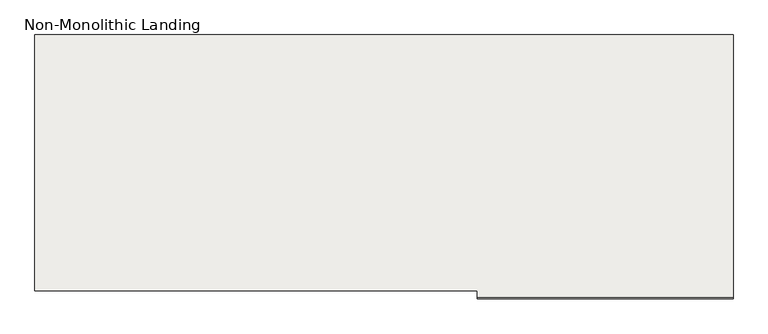
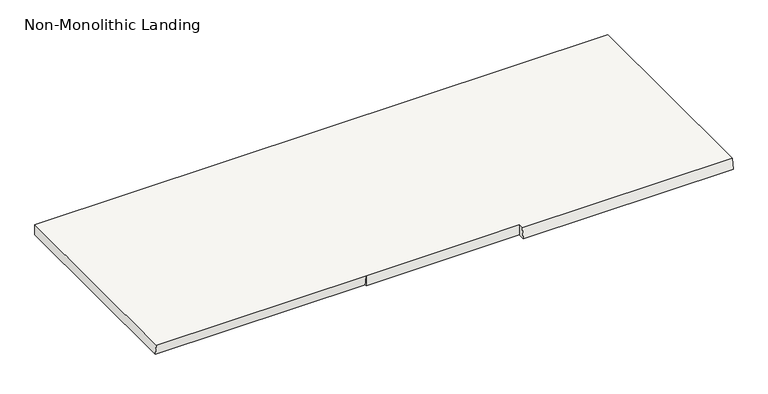
"""IFC4 building model written with IfcOpenShell, lengths in millimetres: slab geometry, Non-Monolithic Landing."""

from ifc_helpers import new_model, si_unit, origin, place, context, project, spatial, faceted_brep, source, transform, mapped, element, save


def non_monolithic_landing_4bf2fde8(model_context):
    return source(origin(), model_context, "Body", "Brep", [
        faceted_brep([(-8867.5141631, 9797.57664, 695.6521739), (-8867.5141631, 9790.38914, 645.6521739), (-7867.4883818, 9790.38914, 645.6521739), (-7867.4883818, 9797.57664, 695.6521739), (-9597.1247141, 9822.57664, 695.6521739), (-8867.5141631, 9822.57664, 695.6521739), (-7867.4883818, 9822.57664, 695.6521739), (-7867.4883818, 10822.6024212, 695.6521739), (-10597.1504953, 10822.6024212, 695.6521739), (-10597.1504953, 9822.57664, 695.6521739), (-8867.5141631, 9822.57664, 645.6521739), (-9597.1247141, 9822.57664, 645.6521739), (-9597.1247141, 9829.76414, 645.6521739), (-10597.1504953, 9829.76414, 645.6521739), (-10597.1504953, 10822.6024212, 645.6521739), (-7867.4883818, 10822.6024212, 645.6521739), (-7867.4883818, 9822.57664, 645.6521739)], [[[0, 1, 2, 3]], [[4, 5, 0, 3, 6, 7, 8, 9]], [[10, 11, 12, 13, 14, 15, 16, 2, 1]], [[5, 4, 11, 10]], [[0, 5, 10, 1]], [[6, 3, 2, 16]], [[7, 6, 16, 15]], [[8, 7, 15, 14]], [[9, 8, 14, 13]], [[4, 12, 11]], [[12, 4, 9, 13]]]),
    ])


if __name__ == "__main__":
    model = new_model("IFC4")
    model_context = context("Model", 3, world=origin())
    ifc_project = project(units=[si_unit("LENGTHUNIT", "METRE", prefix="MILLI")], contexts=[model_context])
    site = spatial("IfcSite", under=ifc_project)
    building = spatial("IfcBuilding", under=site)
    placement = place(None, origin())
    non_monolithic_landing_shape = non_monolithic_landing_4bf2fde8(model_context)
    element("IfcSlab", 1, ObjectType="Non-Monolithic Landing", at=placement, inside=building, context=model_context, shape_type="MappedRepresentation", body=[
        mapped(non_monolithic_landing_shape, transform((0.0, 0.0, 0.0), x_axis=(1.0, 0.0, 0.0), y_axis=(0.0, 1.0, 0.0), z_axis=(0.0, 0.0, 1.0))),
    ])
    save(model, "model.ifc")
